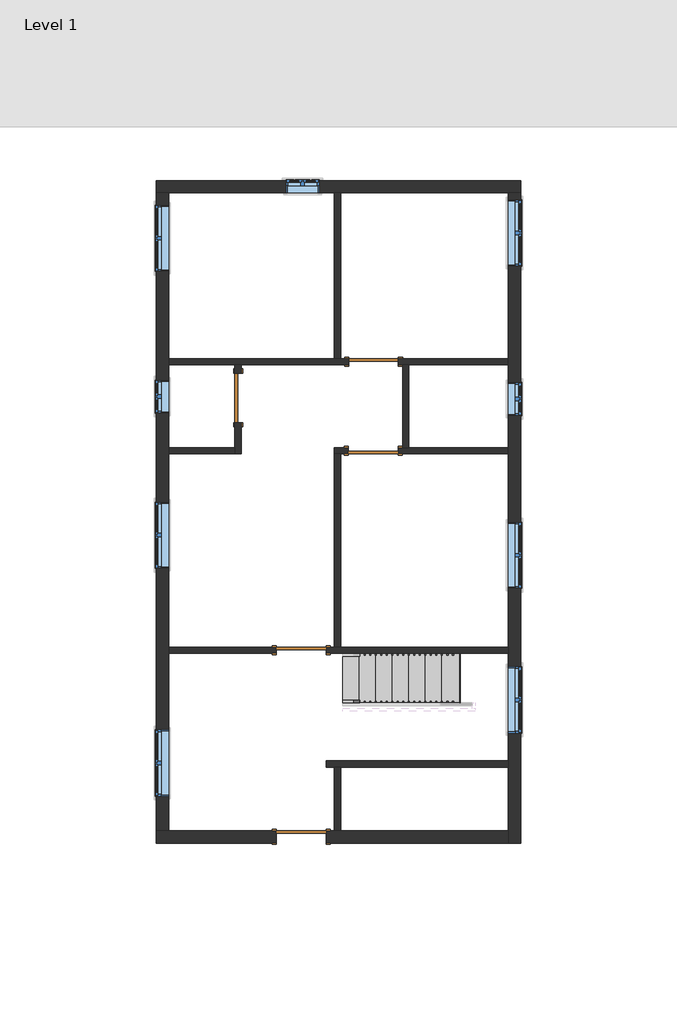
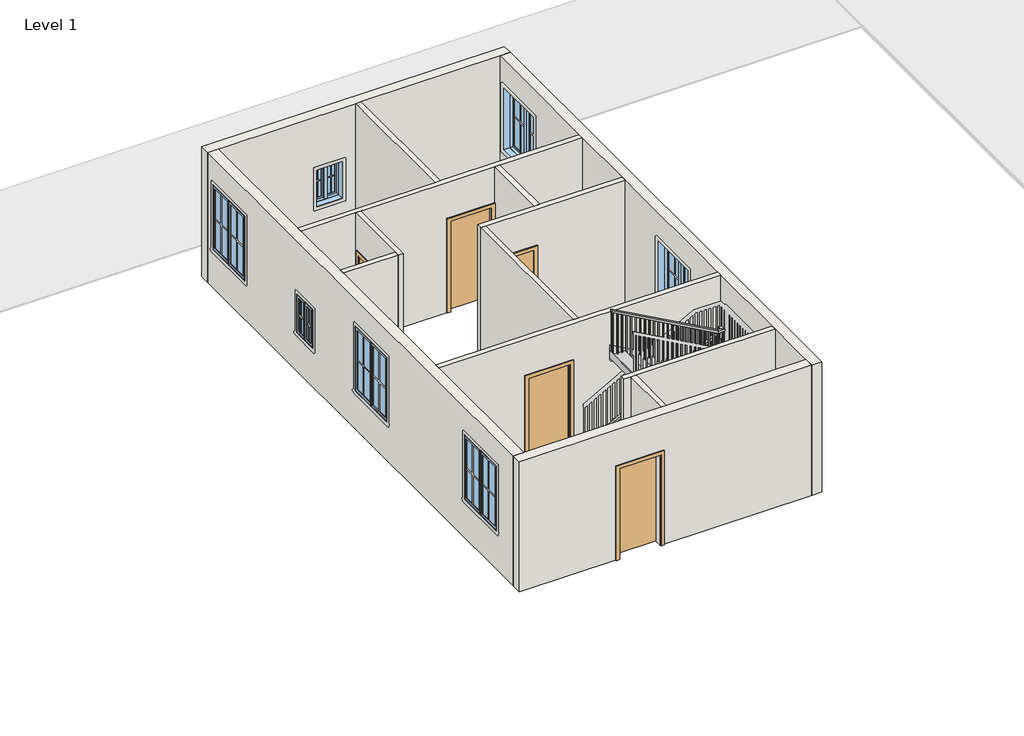
# One storey, part 1 of 2: 14 walls, 9 windows, 5 doors, 1 railing, 1 stair flight.
"""IFC4 building model written with IfcOpenShell, lengths in millimetres."""

from ifc_helpers import new_model, si_unit, frame, origin, origin_with_axes, place, context, project, spatial, polyline, outline, extrude, faceted_brep, transform, mapped, element, save
from components import door_305aa2a5, door_e5f9f3c4, door_a90ba1ad, stair_flight_0ccda8d3, window_c417fced, window_8377141f

model = new_model("IFC4")

# Units and contexts
model_context = context("Model", 3, world=origin())
ifc_project = project(units=[si_unit("LENGTHUNIT", "METRE", prefix="MILLI")], contexts=[model_context])

# Site, building, storey
site = spatial("IfcSite", under=ifc_project)
building = spatial("IfcBuilding", under=site)
storey = spatial("IfcBuildingStorey", under=building, Name="Level 1", Elevation=0.0)

# Doors
placement = place(None, origin())
door_shape = door_305aa2a5(model_context)
element("IfcDoor", 1, ObjectType="Single-Flush : 36\" x 84\"", at=placement, inside=storey, context=model_context, shape_type="MappedRepresentation", body=[
    mapped(door_shape, transform((5270.5, 10636.25, 0.0), x_axis=(-1.0, 0.0, 0.0), y_axis=(0.0, -1.0, 0.0), z_axis=(0.0, 0.0, 1.0))),
])
door_2_shape = door_e5f9f3c4(model_context)
element("IfcDoor", 2, ObjectType="Single-Flush : 36\" x 84\"", at=placement, inside=storey, context=model_context, shape_type="MappedRepresentation", body=[
    mapped(door_2_shape, transform((2774.95, 9969.5, 0.0), x_axis=(0.0, 1.0, 0.0), y_axis=(-1.0, 0.0, 0.0), z_axis=(0.0, 0.0, 1.0))),
])
element("IfcDoor", 3, ObjectType="Single-Flush : 36\" x 84\"", at=placement, inside=storey, context=model_context, shape_type="MappedRepresentation", body=[
    mapped(door_2_shape, transform((5264.15, 8997.95, 0.0), x_axis=(-1.0, 0.0, 0.0), y_axis=(0.0, -1.0, 0.0), z_axis=(0.0, 0.0, 1.0))),
])
element("IfcDoor", 4, ObjectType="Single-Flush : 36\" x 84\"", at=placement, inside=storey, context=model_context, shape_type="MappedRepresentation", body=[
    mapped(door_2_shape, transform((3937.0, 5327.65, 0.0), x_axis=(1.0, 0.0, 0.0), y_axis=(0.0, 1.0, 0.0), z_axis=(0.0, 0.0, 1.0))),
])
door_3_shape = door_a90ba1ad(model_context)
element("IfcDoor", 5, ObjectType="Single-Flush : 36\" x 84\"", at=placement, inside=storey, context=model_context, shape_type="MappedRepresentation", body=[
    mapped(door_3_shape, transform((3937.0, 1892.3, 0.0), x_axis=(-1.0, 0.0, 0.0), y_axis=(0.0, -1.0, 0.0), z_axis=(0.0, 0.0, 1.0))),
])

# Railing
element("IfcRailing", 6, ObjectType="Handrail - Rectangular", at=placement, inside=storey, context=model_context, shape_type="SolidModel", body=[
    faceted_brep([(4699.0, 4406.9, 1083.7333333), (4699.0, 4406.9, 1025.620221), (4699.0, 4356.1, 1025.620221), (4699.0, 4356.1, 1083.7333333), (7061.2, 4406.9, 2396.0666667), (7112.0, 4406.9, 2366.1757765), (7112.0, 4356.1, 2366.1757765), (7061.2, 4356.1, 2396.0666667), (7061.2, 4406.9, 2438.4), (7112.0, 4406.9, 2387.6), (7112.0, 4356.1, 2387.6), (7061.2, 4356.1, 2438.4), (7188.2, 4406.9, 2438.4), (7188.2, 4406.9, 2387.6), (7137.4, 4356.1, 2387.6), (7137.4, 4356.1, 2438.4), (7188.2, 4279.9, 2438.4), (7188.2, 4229.1, 2387.6), (7137.4, 4229.1, 2387.6), (7137.4, 4279.9, 2438.4), (7188.2, 4279.9, 2650.0666667), (7188.2, 4229.1, 2599.2666667), (7137.4, 4229.1, 2599.2666667), (7137.4, 4279.9, 2650.0666667), (7188.2, 4152.9, 2650.0666667), (7188.2, 4152.9, 2599.2666667), (7137.4, 4203.7, 2599.2666667), (7137.4, 4203.7, 2650.0666667), (7061.2, 4152.9, 2650.0666667), (7048.0363978, 4152.9, 2599.2666667), (7048.0363978, 4203.7, 2599.2666667), (7061.2, 4203.7, 2650.0666667), (4699.0, 4152.9, 3962.4), (4699.0, 4203.7, 3962.4), (4699.0, 4203.7, 3904.2868876), (4699.0, 4152.9, 3904.2868876)], [[[0, 1, 2, 3]], [[1, 0, 4, 5]], [[2, 1, 5, 6]], [[3, 2, 6, 7]], [[0, 3, 7, 4]], [[5, 4, 8, 9]], [[6, 5, 9, 10]], [[7, 6, 10, 11]], [[4, 7, 11, 8]], [[9, 8, 12, 13]], [[10, 9, 13, 14]], [[11, 10, 14, 15]], [[8, 11, 15, 12]], [[13, 12, 16, 17]], [[14, 13, 17, 18]], [[15, 14, 18, 19]], [[12, 15, 19, 16]], [[17, 16, 20, 21]], [[18, 17, 21, 22]], [[19, 18, 22, 23]], [[16, 19, 23, 20]], [[21, 20, 24, 25]], [[22, 21, 25, 26]], [[23, 22, 26, 27]], [[20, 23, 27, 24]], [[25, 24, 28, 29]], [[26, 25, 29, 30]], [[27, 26, 30, 31]], [[24, 27, 31, 28]], [[32, 33, 34, 35]], [[29, 28, 32, 35]], [[30, 29, 35, 34]], [[31, 30, 34, 33]], [[28, 31, 33, 32]]]),
    extrude(outline(polyline([(3884.8841099, 4733.925), (3895.4674432, 4714.875), (2878.6666667, 4714.875), (2878.6666667, 4733.925), (3884.8841099, 4733.925)])), frame((0.0, 4168.775, 0.0), z_axis=(0.0, 1.0, 0.0), x_axis=(0.0, 0.0, 1.0)), (0.0, 0.0, 1.0), 19.05),
    extrude(outline(polyline([(3828.4396654, 4835.525), (3839.0229988, 4816.475), (2878.6666667, 4816.475), (2878.6666667, 4835.525), (3828.4396654, 4835.525)])), frame((0.0, 4168.775, 0.0), z_axis=(0.0, 1.0, 0.0), x_axis=(0.0, 0.0, 1.0)), (0.0, 0.0, 1.0), 19.05),
    extrude(outline(polyline([(3771.995221, 4937.125), (3782.5785543, 4918.075), (2878.6666667, 4918.075), (2878.6666667, 4937.125), (3771.995221, 4937.125)])), frame((0.0, 4168.775, 0.0), z_axis=(0.0, 1.0, 0.0), x_axis=(0.0, 0.0, 1.0)), (0.0, 0.0, 1.0), 19.05),
    extrude(outline(polyline([(3715.5507765, 5038.725), (3726.1341099, 5019.675), (2709.3333333, 5019.675), (2709.3333333, 5038.725), (3715.5507765, 5038.725)])), frame((0.0, 4168.775, 0.0), z_axis=(0.0, 1.0, 0.0), x_axis=(0.0, 0.0, 1.0)), (0.0, 0.0, 1.0), 19.05),
    extrude(outline(polyline([(3659.1063321, 5140.325), (3669.6896654, 5121.275), (2709.3333333, 5121.275), (2709.3333333, 5140.325), (3659.1063321, 5140.325)])), frame((0.0, 4168.775, 0.0), z_axis=(0.0, 1.0, 0.0), x_axis=(0.0, 0.0, 1.0)), (0.0, 0.0, 1.0), 19.05),
    extrude(outline(polyline([(3602.6618876, 5241.925), (3613.245221, 5222.875), (2709.3333333, 5222.875), (2709.3333333, 5241.925), (3602.6618876, 5241.925)])), frame((0.0, 4168.775, 0.0), z_axis=(0.0, 1.0, 0.0), x_axis=(0.0, 0.0, 1.0)), (0.0, 0.0, 1.0), 19.05),
    extrude(outline(polyline([(3546.2174432, 5343.525), (3556.8007765, 5324.475), (2540.0, 5324.475), (2540.0, 5343.525), (3546.2174432, 5343.525)])), frame((0.0, 4168.775, 0.0), z_axis=(0.0, 1.0, 0.0), x_axis=(0.0, 0.0, 1.0)), (0.0, 0.0, 1.0), 19.05),
    extrude(outline(polyline([(3489.7729988, 5445.125), (3500.3563321, 5426.075), (2540.0, 5426.075), (2540.0, 5445.125), (3489.7729988, 5445.125)])), frame((0.0, 4168.775, 0.0), z_axis=(0.0, 1.0, 0.0), x_axis=(0.0, 0.0, 1.0)), (0.0, 0.0, 1.0), 19.05),
    extrude(outline(polyline([(3433.3285543, 5546.725), (3443.9118876, 5527.675), (2540.0, 5527.675), (2540.0, 5546.725), (3433.3285543, 5546.725)])), frame((0.0, 4168.775, 0.0), z_axis=(0.0, 1.0, 0.0), x_axis=(0.0, 0.0, 1.0)), (0.0, 0.0, 1.0), 19.05),
    extrude(outline(polyline([(3376.8841099, 5648.325), (3387.4674432, 5629.275), (2370.6666667, 5629.275), (2370.6666667, 5648.325), (3376.8841099, 5648.325)])), frame((0.0, 4168.775, 0.0), z_axis=(0.0, 1.0, 0.0), x_axis=(0.0, 0.0, 1.0)), (0.0, 0.0, 1.0), 19.05),
    extrude(outline(polyline([(3320.4396654, 5749.925), (3331.0229988, 5730.875), (2370.6666667, 5730.875), (2370.6666667, 5749.925), (3320.4396654, 5749.925)])), frame((0.0, 4168.775, 0.0), z_axis=(0.0, 1.0, 0.0), x_axis=(0.0, 0.0, 1.0)), (0.0, 0.0, 1.0), 19.05),
    extrude(outline(polyline([(3263.995221, 5851.525), (3274.5785543, 5832.475), (2370.6666667, 5832.475), (2370.6666667, 5851.525), (3263.995221, 5851.525)])), frame((0.0, 4168.775, 0.0), z_axis=(0.0, 1.0, 0.0), x_axis=(0.0, 0.0, 1.0)), (0.0, 0.0, 1.0), 19.05),
    extrude(outline(polyline([(3207.5507765, 5953.125), (3218.1341099, 5934.075), (2201.3333333, 5934.075), (2201.3333333, 5953.125), (3207.5507765, 5953.125)])), frame((0.0, 4168.775, 0.0), z_axis=(0.0, 1.0, 0.0), x_axis=(0.0, 0.0, 1.0)), (0.0, 0.0, 1.0), 19.05),
    extrude(outline(polyline([(3151.1063321, 6054.725), (3161.6896654, 6035.675), (2201.3333333, 6035.675), (2201.3333333, 6054.725), (3151.1063321, 6054.725)])), frame((0.0, 4168.775, 0.0), z_axis=(0.0, 1.0, 0.0), x_axis=(0.0, 0.0, 1.0)), (0.0, 0.0, 1.0), 19.05),
    extrude(outline(polyline([(3094.6618876, 6156.325), (3105.245221, 6137.275), (2201.3333333, 6137.275), (2201.3333333, 6156.325), (3094.6618876, 6156.325)])), frame((0.0, 4168.775, 0.0), z_axis=(0.0, 1.0, 0.0), x_axis=(0.0, 0.0, 1.0)), (0.0, 0.0, 1.0), 19.05),
    extrude(outline(polyline([(3038.2174432, 6257.925), (3048.8007765, 6238.875), (2032.0, 6238.875), (2032.0, 6257.925), (3038.2174432, 6257.925)])), frame((0.0, 4168.775, 0.0), z_axis=(0.0, 1.0, 0.0), x_axis=(0.0, 0.0, 1.0)), (0.0, 0.0, 1.0), 19.05),
    extrude(outline(polyline([(2981.7729988, 6359.525), (2992.3563321, 6340.475), (2032.0, 6340.475), (2032.0, 6359.525), (2981.7729988, 6359.525)])), frame((0.0, 4168.775, 0.0), z_axis=(0.0, 1.0, 0.0), x_axis=(0.0, 0.0, 1.0)), (0.0, 0.0, 1.0), 19.05),
    extrude(outline(polyline([(2925.3285543, 6461.125), (2935.9118876, 6442.075), (2032.0, 6442.075), (2032.0, 6461.125), (2925.3285543, 6461.125)])), frame((0.0, 4168.775, 0.0), z_axis=(0.0, 1.0, 0.0), x_axis=(0.0, 0.0, 1.0)), (0.0, 0.0, 1.0), 19.05),
    extrude(outline(polyline([(2868.8841099, 6562.725), (2879.4674432, 6543.675), (1862.6666667, 6543.675), (1862.6666667, 6562.725), (2868.8841099, 6562.725)])), frame((0.0, 4168.775, 0.0), z_axis=(0.0, 1.0, 0.0), x_axis=(0.0, 0.0, 1.0)), (0.0, 0.0, 1.0), 19.05),
    extrude(outline(polyline([(2812.4396654, 6664.325), (2823.0229988, 6645.275), (1862.6666667, 6645.275), (1862.6666667, 6664.325), (2812.4396654, 6664.325)])), frame((0.0, 4168.775, 0.0), z_axis=(0.0, 1.0, 0.0), x_axis=(0.0, 0.0, 1.0)), (0.0, 0.0, 1.0), 19.05),
    extrude(outline(polyline([(2755.995221, 6765.925), (2766.5785543, 6746.875), (1862.6666667, 6746.875), (1862.6666667, 6765.925), (2755.995221, 6765.925)])), frame((0.0, 4168.775, 0.0), z_axis=(0.0, 1.0, 0.0), x_axis=(0.0, 0.0, 1.0)), (0.0, 0.0, 1.0), 19.05),
    extrude(outline(polyline([(2699.5507765, 6867.525), (2710.1341099, 6848.475), (1693.3333333, 6848.475), (1693.3333333, 6867.525), (2699.5507765, 6867.525)])), frame((0.0, 4168.775, 0.0), z_axis=(0.0, 1.0, 0.0), x_axis=(0.0, 0.0, 1.0)), (0.0, 0.0, 1.0), 19.05),
    extrude(outline(polyline([(2643.1063321, 6969.125), (2653.6896654, 6950.075), (1693.3333333, 6950.075), (1693.3333333, 6969.125), (2643.1063321, 6969.125)])), frame((0.0, 4168.775, 0.0), z_axis=(0.0, 1.0, 0.0), x_axis=(0.0, 0.0, 1.0)), (0.0, 0.0, 1.0), 19.05),
    extrude(outline(polyline([(2586.6618876, 7070.725), (2597.245221, 7051.675), (1693.3333333, 7051.675), (1693.3333333, 7070.725), (2586.6618876, 7070.725)])), frame((0.0, 4168.775, 0.0), z_axis=(0.0, 1.0, 0.0), x_axis=(0.0, 0.0, 1.0)), (0.0, 0.0, 1.0), 19.05),
    extrude(outline(polyline([(7153.275, 4289.425), (7172.325, 4289.425), (7172.325, 4270.375), (7153.275, 4270.375), (7153.275, 4289.425)])), frame((0.0, 0.0, 1524.0), z_axis=(0.0, 0.0, 1.0), x_axis=(1.0, 0.0, 0.0)), (0.0, 0.0, 1.0), 863.6),
    extrude(outline(polyline([(7127.875, 4371.975), (7127.875, 4391.025), (7146.925, 4391.025), (7146.925, 4371.975), (7127.875, 4371.975)])), frame((0.0, 0.0, 1524.0), z_axis=(0.0, 0.0, 1.0), x_axis=(1.0, 0.0, 0.0)), (0.0, 0.0, 1.0), 863.6),
    extrude(outline(polyline([(2329.1341099, 7045.325), (2318.5507765, 7026.275), (1354.6666667, 7026.275), (1354.6666667, 7045.325), (2329.1341099, 7045.325)])), frame((0.0, 4371.975, 0.0), z_axis=(0.0, 1.0, 0.0), x_axis=(0.0, 0.0, 1.0)), (0.0, 0.0, 1.0), 19.05),
    extrude(outline(polyline([(2272.6896654, 6943.725), (2262.1063321, 6924.675), (1354.6666667, 6924.675), (1354.6666667, 6943.725), (2272.6896654, 6943.725)])), frame((0.0, 4371.975, 0.0), z_axis=(0.0, 1.0, 0.0), x_axis=(0.0, 0.0, 1.0)), (0.0, 0.0, 1.0), 19.05),
    extrude(outline(polyline([(2216.245221, 6842.125), (2205.6618876, 6823.075), (1354.6666667, 6823.075), (1354.6666667, 6842.125), (2216.245221, 6842.125)])), frame((0.0, 4371.975, 0.0), z_axis=(0.0, 1.0, 0.0), x_axis=(0.0, 0.0, 1.0)), (0.0, 0.0, 1.0), 19.05),
    extrude(outline(polyline([(2159.8007765, 6740.525), (2149.2174432, 6721.475), (1185.3333333, 6721.475), (1185.3333333, 6740.525), (2159.8007765, 6740.525)])), frame((0.0, 4371.975, 0.0), z_axis=(0.0, 1.0, 0.0), x_axis=(0.0, 0.0, 1.0)), (0.0, 0.0, 1.0), 19.05),
    extrude(outline(polyline([(2103.3563321, 6638.925), (2092.7729988, 6619.875), (1185.3333333, 6619.875), (1185.3333333, 6638.925), (2103.3563321, 6638.925)])), frame((0.0, 4371.975, 0.0), z_axis=(0.0, 1.0, 0.0), x_axis=(0.0, 0.0, 1.0)), (0.0, 0.0, 1.0), 19.05),
    extrude(outline(polyline([(2046.9118876, 6537.325), (2036.3285543, 6518.275), (1185.3333333, 6518.275), (1185.3333333, 6537.325), (2046.9118876, 6537.325)])), frame((0.0, 4371.975, 0.0), z_axis=(0.0, 1.0, 0.0), x_axis=(0.0, 0.0, 1.0)), (0.0, 0.0, 1.0), 19.05),
    extrude(outline(polyline([(1990.4674432, 6435.725), (1979.8841099, 6416.675), (1016.0, 6416.675), (1016.0, 6435.725), (1990.4674432, 6435.725)])), frame((0.0, 4371.975, 0.0), z_axis=(0.0, 1.0, 0.0), x_axis=(0.0, 0.0, 1.0)), (0.0, 0.0, 1.0), 19.05),
    extrude(outline(polyline([(1934.0229988, 6334.125), (1923.4396654, 6315.075), (1016.0, 6315.075), (1016.0, 6334.125), (1934.0229988, 6334.125)])), frame((0.0, 4371.975, 0.0), z_axis=(0.0, 1.0, 0.0), x_axis=(0.0, 0.0, 1.0)), (0.0, 0.0, 1.0), 19.05),
    extrude(outline(polyline([(1877.5785543, 6232.525), (1866.995221, 6213.475), (1016.0, 6213.475), (1016.0, 6232.525), (1877.5785543, 6232.525)])), frame((0.0, 4371.975, 0.0), z_axis=(0.0, 1.0, 0.0), x_axis=(0.0, 0.0, 1.0)), (0.0, 0.0, 1.0), 19.05),
    extrude(outline(polyline([(1821.1341099, 6130.925), (1810.5507765, 6111.875), (846.6666667, 6111.875), (846.6666667, 6130.925), (1821.1341099, 6130.925)])), frame((0.0, 4371.975, 0.0), z_axis=(0.0, 1.0, 0.0), x_axis=(0.0, 0.0, 1.0)), (0.0, 0.0, 1.0), 19.05),
    extrude(outline(polyline([(1764.6896654, 6029.325), (1754.1063321, 6010.275), (846.6666667, 6010.275), (846.6666667, 6029.325), (1764.6896654, 6029.325)])), frame((0.0, 4371.975, 0.0), z_axis=(0.0, 1.0, 0.0), x_axis=(0.0, 0.0, 1.0)), (0.0, 0.0, 1.0), 19.05),
    extrude(outline(polyline([(1708.245221, 5927.725), (1697.6618876, 5908.675), (846.6666667, 5908.675), (846.6666667, 5927.725), (1708.245221, 5927.725)])), frame((0.0, 4371.975, 0.0), z_axis=(0.0, 1.0, 0.0), x_axis=(0.0, 0.0, 1.0)), (0.0, 0.0, 1.0), 19.05),
    extrude(outline(polyline([(1651.8007765, 5826.125), (1641.2174432, 5807.075), (677.3333333, 5807.075), (677.3333333, 5826.125), (1651.8007765, 5826.125)])), frame((0.0, 4371.975, 0.0), z_axis=(0.0, 1.0, 0.0), x_axis=(0.0, 0.0, 1.0)), (0.0, 0.0, 1.0), 19.05),
    extrude(outline(polyline([(1595.3563321, 5724.525), (1584.7729988, 5705.475), (677.3333333, 5705.475), (677.3333333, 5724.525), (1595.3563321, 5724.525)])), frame((0.0, 4371.975, 0.0), z_axis=(0.0, 1.0, 0.0), x_axis=(0.0, 0.0, 1.0)), (0.0, 0.0, 1.0), 19.05),
    extrude(outline(polyline([(1538.9118876, 5622.925), (1528.3285543, 5603.875), (677.3333333, 5603.875), (677.3333333, 5622.925), (1538.9118876, 5622.925)])), frame((0.0, 4371.975, 0.0), z_axis=(0.0, 1.0, 0.0), x_axis=(0.0, 0.0, 1.0)), (0.0, 0.0, 1.0), 19.05),
    extrude(outline(polyline([(1482.4674432, 5521.325), (1471.8841099, 5502.275), (508.0, 5502.275), (508.0, 5521.325), (1482.4674432, 5521.325)])), frame((0.0, 4371.975, 0.0), z_axis=(0.0, 1.0, 0.0), x_axis=(0.0, 0.0, 1.0)), (0.0, 0.0, 1.0), 19.05),
    extrude(outline(polyline([(1426.0229988, 5419.725), (1415.4396654, 5400.675), (508.0, 5400.675), (508.0, 5419.725), (1426.0229988, 5419.725)])), frame((0.0, 4371.975, 0.0), z_axis=(0.0, 1.0, 0.0), x_axis=(0.0, 0.0, 1.0)), (0.0, 0.0, 1.0), 19.05),
    extrude(outline(polyline([(1369.5785543, 5318.125), (1358.995221, 5299.075), (508.0, 5299.075), (508.0, 5318.125), (1369.5785543, 5318.125)])), frame((0.0, 4371.975, 0.0), z_axis=(0.0, 1.0, 0.0), x_axis=(0.0, 0.0, 1.0)), (0.0, 0.0, 1.0), 19.05),
    extrude(outline(polyline([(1313.1341099, 5216.525), (1302.5507765, 5197.475), (338.6666667, 5197.475), (338.6666667, 5216.525), (1313.1341099, 5216.525)])), frame((0.0, 4371.975, 0.0), z_axis=(0.0, 1.0, 0.0), x_axis=(0.0, 0.0, 1.0)), (0.0, 0.0, 1.0), 19.05),
    extrude(outline(polyline([(1256.6896654, 5114.925), (1246.1063321, 5095.875), (338.6666667, 5095.875), (338.6666667, 5114.925), (1256.6896654, 5114.925)])), frame((0.0, 4371.975, 0.0), z_axis=(0.0, 1.0, 0.0), x_axis=(0.0, 0.0, 1.0)), (0.0, 0.0, 1.0), 19.05),
    extrude(outline(polyline([(1200.245221, 5013.325), (1189.6618876, 4994.275), (338.6666667, 4994.275), (338.6666667, 5013.325), (1200.245221, 5013.325)])), frame((0.0, 4371.975, 0.0), z_axis=(0.0, 1.0, 0.0), x_axis=(0.0, 0.0, 1.0)), (0.0, 0.0, 1.0), 19.05),
    extrude(outline(polyline([(1143.8007765, 4911.725), (1133.2174432, 4892.675), (169.3333333, 4892.675), (169.3333333, 4911.725), (1143.8007765, 4911.725)])), frame((0.0, 4371.975, 0.0), z_axis=(0.0, 1.0, 0.0), x_axis=(0.0, 0.0, 1.0)), (0.0, 0.0, 1.0), 19.05),
    extrude(outline(polyline([(1087.3563321, 4810.125), (1076.7729988, 4791.075), (169.3333333, 4791.075), (169.3333333, 4810.125), (1087.3563321, 4810.125)])), frame((0.0, 4371.975, 0.0), z_axis=(0.0, 1.0, 0.0), x_axis=(0.0, 0.0, 1.0)), (0.0, 0.0, 1.0), 19.05),
    extrude(outline(polyline([(7153.275, 4187.825), (7172.325, 4187.825), (7172.325, 4168.775), (7153.275, 4168.775), (7153.275, 4187.825)])), frame((0.0, 0.0, 1524.0), z_axis=(0.0, 0.0, 1.0), x_axis=(1.0, 0.0, 0.0)), (0.0, 0.0, 1.0), 1075.2666667),
    extrude(outline(polyline([(7153.275, 4371.975), (7153.275, 4391.025), (7172.325, 4391.025), (7172.325, 4371.975), (7153.275, 4371.975)])), frame((0.0, 0.0, 1524.0), z_axis=(0.0, 0.0, 1.0), x_axis=(1.0, 0.0, 0.0)), (0.0, 0.0, 1.0), 863.6),
    extrude(outline(polyline([(3893.7035543, 4718.05), (3904.2868876, 4699.0), (2878.6666667, 4699.0), (2878.6666667, 4718.05), (3893.7035543, 4718.05)])), frame((0.0, 4168.775, 0.0), z_axis=(0.0, 1.0, 0.0), x_axis=(0.0, 0.0, 1.0)), (0.0, 0.0, 1.0), 19.05),
    extrude(outline(polyline([(1036.2035543, 4718.05), (1025.620221, 4699.0), (169.3333333, 4699.0), (169.3333333, 4718.05), (1036.2035543, 4718.05)])), frame((0.0, 4371.975, 0.0), z_axis=(0.0, 1.0, 0.0), x_axis=(0.0, 0.0, 1.0)), (0.0, 0.0, 1.0), 19.05),
])

# Stair flight
stair_flight_shape = stair_flight_0ccda8d3(model_context)
element("IfcStairFlight", 7, ObjectType="2\" Tread 1\" Nosing 1/4\" Riser", at=placement, inside=storey, context=model_context, shape_type="MappedRepresentation", body=[
    mapped(stair_flight_shape, transform((0.0, 0.0, 0.0), x_axis=(1.0, 0.0, 0.0), y_axis=(0.0, 1.0, 0.0), z_axis=(0.0, 0.0, 1.0))),
])

# Walls
element("IfcWall", 8, ObjectType="Generic - 5\"", at=placement, inside=storey, context=model_context, shape_type="SweptSolid", body=[
    extrude(outline(polyline([(4546.6, 10693.4), (4546.6, 13741.4), (4660.9, 13741.4), (4660.9, 10693.4), (4546.6, 10693.4)])), origin_with_axes(), (0.0, 0.0, 1.0), 3048.0),
])
element("IfcWall", 9, ObjectType="Generic - 5\"", at=placement, inside=storey, context=model_context, shape_type="Brep", body=[
    faceted_brep([(1498.6, 10579.1, 0.0), (2717.8, 10579.1, 0.0), (2832.1, 10579.1, 0.0), (4813.3, 10579.1, 0.0), (4813.3, 10579.1, 2133.6), (5727.7, 10579.1, 2133.6), (5727.7, 10579.1, 0.0), (5803.9, 10579.1, 0.0), (5918.2, 10579.1, 0.0), (7747.0, 10579.1, 0.0), (7747.0, 10579.1, 3048.0), (5918.2, 10579.1, 3048.0), (5803.9, 10579.1, 3048.0), (2832.1, 10579.1, 3048.0), (2717.8, 10579.1, 3048.0), (1498.6, 10579.1, 3048.0), (4813.3, 10693.4, 2133.6), (4813.3, 10693.4, 0.0), (4660.9, 10693.4, 0.0), (4546.6, 10693.4, 0.0), (1498.6, 10693.4, 0.0), (1498.6, 10693.4, 3048.0), (4546.6, 10693.4, 3048.0), (4660.9, 10693.4, 3048.0), (7747.0, 10693.4, 3048.0), (7747.0, 10693.4, 0.0), (5727.7, 10693.4, 0.0), (5727.7, 10693.4, 2133.6)], [[[0, 1, 2, 3, 4, 5, 6, 7, 8, 9, 10, 11, 12, 13, 14, 15]], [[16, 17, 18, 19, 20, 21, 22, 23, 24, 25, 26, 27]], [[26, 25, 9, 8, 7, 6]], [[20, 19, 18, 17, 3, 2, 1, 0]], [[15, 14, 13, 12, 11, 10, 24, 23, 22, 21]], [[10, 9, 25, 24]], [[0, 15, 21, 20]], [[4, 3, 17, 16]], [[5, 4, 16, 27]], [[6, 5, 27, 26]]]),
])
element("IfcWall", 10, ObjectType="Generic - 5\"", at=placement, inside=storey, context=model_context, shape_type="Brep", body=[
    faceted_brep([(2717.8, 10579.1, 0.0), (2717.8, 10426.7, 0.0), (2717.8, 10426.7, 2133.6), (2717.8, 9512.3, 2133.6), (2717.8, 9512.3, 0.0), (2717.8, 9055.1, 0.0), (2717.8, 8940.8, 0.0), (2717.8, 8940.8, 3048.0), (2717.8, 9055.1, 3048.0), (2717.8, 10579.1, 3048.0), (2832.1, 10426.7, 2133.6), (2832.1, 10426.7, 0.0), (2832.1, 10579.1, 0.0), (2832.1, 10579.1, 3048.0), (2832.1, 8940.8, 3048.0), (2832.1, 8940.8, 0.0), (2832.1, 9512.3, 0.0), (2832.1, 9512.3, 2133.6)], [[[0, 1, 2, 3, 4, 5, 6, 7, 8, 9]], [[10, 11, 12, 13, 14, 15, 16, 17]], [[16, 15, 6, 5, 4]], [[12, 11, 1, 0]], [[9, 8, 7, 14, 13]], [[0, 9, 13, 12]], [[7, 6, 15, 14]], [[2, 1, 11, 10]], [[3, 2, 10, 17]], [[4, 3, 17, 16]]]),
])
element("IfcWall", 11, ObjectType="Generic - 5\"", at=placement, inside=storey, context=model_context, shape_type="SweptSolid", body=[
    extrude(outline(polyline([(2717.8, 8940.8), (1498.6, 8940.8), (1498.6, 9055.1), (2717.8, 9055.1), (2717.8, 8940.8)])), origin_with_axes(), (0.0, 0.0, 1.0), 3048.0),
])
element("IfcWall", 12, ObjectType="Generic - 5\"", at=placement, inside=storey, context=model_context, shape_type="SweptSolid", body=[
    extrude(outline(polyline([(5803.9, 9055.1), (5803.9, 10579.1), (5918.2, 10579.1), (5918.2, 9055.1), (5803.9, 9055.1)])), origin_with_axes(), (0.0, 0.0, 1.0), 3048.0),
])
element("IfcWall", 13, ObjectType="Generic - 5\"", at=placement, inside=storey, context=model_context, shape_type="Brep", body=[
    faceted_brep([(4806.95, 9055.1, 2133.6), (4806.95, 9055.1, 0.0), (4546.6, 9055.1, 0.0), (4546.6, 9055.1, 3048.0), (5803.9, 9055.1, 3048.0), (5918.2, 9055.1, 3048.0), (7747.0, 9055.1, 3048.0), (7747.0, 9055.1, 0.0), (5918.2, 9055.1, 0.0), (5803.9, 9055.1, 0.0), (5721.35, 9055.1, 0.0), (5721.35, 9055.1, 2133.6), (4546.6, 8940.8, 0.0), (4660.9, 8940.8, 0.0), (4806.95, 8940.8, 0.0), (4806.95, 8940.8, 2133.6), (5721.35, 8940.8, 2133.6), (5721.35, 8940.8, 0.0), (7747.0, 8940.8, 0.0), (7747.0, 8940.8, 3048.0), (4660.9, 8940.8, 3048.0), (4546.6, 8940.8, 3048.0)], [[[0, 1, 2, 3, 4, 5, 6, 7, 8, 9, 10, 11]], [[12, 13, 14, 15, 16, 17, 18, 19, 20, 21]], [[2, 1, 14, 13, 12]], [[10, 9, 8, 7, 18, 17]], [[6, 5, 4, 3, 21, 20, 19]], [[7, 6, 19, 18]], [[3, 2, 12, 21]], [[15, 14, 1, 0]], [[16, 15, 0, 11]], [[17, 16, 11, 10]]]),
])
element("IfcWall", 14, ObjectType="Generic - 5\"", at=placement, inside=storey, context=model_context, shape_type="Brep", body=[
    faceted_brep([(4394.2, 5270.5, 2133.6), (4394.2, 5270.5, 0.0), (7747.0, 5270.5, 0.0), (7747.0, 5270.5, 3048.0), (1498.6, 5270.5, 3048.0), (1498.6, 5270.5, 0.0), (3479.8, 5270.5, 0.0), (3479.8, 5270.5, 2133.6), (7747.0, 5384.8, 0.0), (4660.9, 5384.8, 0.0), (4546.6, 5384.8, 0.0), (4394.2, 5384.8, 0.0), (4394.2, 5384.8, 2133.6), (3479.8, 5384.8, 2133.6), (3479.8, 5384.8, 0.0), (1498.6, 5384.8, 0.0), (1498.6, 5384.8, 3048.0), (4546.6, 5384.8, 3048.0), (4660.9, 5384.8, 3048.0), (7747.0, 5384.8, 3048.0)], [[[0, 1, 2, 3, 4, 5, 6, 7]], [[8, 9, 10, 11, 12, 13, 14, 15, 16, 17, 18, 19]], [[6, 5, 15, 14]], [[2, 1, 11, 10, 9, 8]], [[4, 3, 19, 18, 17, 16]], [[3, 2, 8, 19]], [[5, 4, 16, 15]], [[12, 11, 1, 0]], [[13, 12, 0, 7]], [[14, 13, 7, 6]]]),
])
element("IfcWall", 15, ObjectType="Generic - 5\"", at=placement, inside=storey, context=model_context, shape_type="SweptSolid", body=[
    extrude(outline(polyline([(4660.9, 8940.8), (4660.9, 5384.8), (4546.6, 5384.8), (4546.6, 8940.8), (4660.9, 8940.8)])), origin_with_axes(), (0.0, 0.0, 1.0), 3048.0),
])
element("IfcWall", 16, ObjectType="Generic - 5\"", at=placement, inside=storey, context=model_context, shape_type="SweptSolid", body=[
    extrude(outline(polyline([(4660.9, 3175.0), (4660.9, 2006.6), (4546.6, 2006.6), (4546.6, 3175.0), (4660.9, 3175.0)])), origin_with_axes(), (0.0, 0.0, 1.0), 3048.0),
])
element("IfcWall", 17, ObjectType="Generic - 5\"", at=placement, inside=storey, context=model_context, shape_type="Brep", body=[
    faceted_brep([(4394.2, 3175.0, 0.0), (4546.6, 3175.0, 0.0), (4660.9, 3175.0, 0.0), (7747.0, 3175.0, 0.0), (7747.0, 3175.0, 3048.0), (4660.9, 3175.0, 3048.0), (4546.6, 3175.0, 3048.0), (4394.2, 3175.0, 3048.0), (4394.2, 3289.3, 0.0), (4394.2, 3289.3, 3048.0), (7747.0, 3289.3, 3048.0), (7747.0, 3289.3, 0.0)], [[[0, 1, 2, 3, 4, 5, 6, 7]], [[8, 9, 10, 11]], [[3, 2, 1, 0, 8, 11]], [[7, 6, 5, 4, 10, 9]], [[0, 7, 9, 8]], [[4, 3, 11, 10]]]),
])
element("IfcWall", 18, ObjectType="Generic - 8\"", at=placement, inside=storey, context=model_context, shape_type="Brep", body=[
    faceted_brep([(1270.0, 13741.4, 0.0), (1498.6, 13741.4, 0.0), (4546.6, 13741.4, 0.0), (4660.9, 13741.4, 0.0), (7747.0, 13741.4, 0.0), (7975.6, 13741.4, 0.0), (7975.6, 13741.4, 3048.0), (7747.0, 13741.4, 3048.0), (4660.9, 13741.4, 3048.0), (4546.6, 13741.4, 3048.0), (1498.6, 13741.4, 3048.0), (1270.0, 13741.4, 3048.0), (4267.2, 13741.4, 1828.8), (4267.2, 13741.4, 914.4), (3657.6, 13741.4, 914.4), (3657.6, 13741.4, 1828.8), (1270.0, 13970.0, 0.0), (1270.0, 13970.0, 3048.0), (7975.6, 13970.0, 3048.0), (7975.6, 13970.0, 0.0), (4267.2, 13970.0, 1828.8), (3657.6, 13970.0, 1828.8), (3657.6, 13970.0, 914.4), (4267.2, 13970.0, 914.4)], [[[0, 1, 2, 3, 4, 5, 6, 7, 8, 9, 10, 11], [12, 13, 14, 15]], [[16, 17, 18, 19], [20, 21, 22, 23]], [[5, 4, 3, 2, 1, 0, 16, 19]], [[6, 5, 19, 18]], [[0, 11, 17, 16]], [[13, 12, 20, 23]], [[14, 13, 23, 22]], [[15, 14, 22, 21]], [[12, 15, 21, 20]], [[11, 10, 9, 8, 7, 6, 18, 17]]]),
])
element("IfcWall", 19, ObjectType="Generic - 8\"", at=placement, inside=storey, context=model_context, shape_type="Brep", body=[
    faceted_brep([(7747.0, 13741.4, 0.0), (7747.0, 10693.4, 0.0), (7747.0, 10579.1, 0.0), (7747.0, 9055.1, 0.0), (7747.0, 8940.8, 0.0), (7747.0, 5384.8, 0.0), (7747.0, 5270.5, 0.0), (7747.0, 3289.3, 0.0), (7747.0, 3175.0, 0.0), (7747.0, 2006.6, 0.0), (7747.0, 1778.0, 0.0), (7747.0, 1778.0, 3048.0), (7747.0, 2006.6, 3048.0), (7747.0, 3175.0, 3048.0), (7747.0, 3289.3, 3048.0), (7747.0, 5270.5, 3048.0), (7747.0, 5384.8, 3048.0), (7747.0, 8940.8, 3048.0), (7747.0, 9055.1, 3048.0), (7747.0, 10579.1, 3048.0), (7747.0, 10693.4, 3048.0), (7747.0, 13741.4, 3048.0), (7747.0, 12395.2, 2438.4), (7747.0, 12395.2, 914.4), (7747.0, 13614.4, 914.4), (7747.0, 13614.4, 2438.4), (7747.0, 6464.3, 2438.4), (7747.0, 6464.3, 914.4), (7747.0, 7683.5, 914.4), (7747.0, 7683.5, 2438.4), (7747.0, 9645.65, 1828.8), (7747.0, 9645.65, 914.4), (7747.0, 10255.25, 914.4), (7747.0, 10255.25, 1828.8), (7747.0, 3803.65, 2438.4), (7747.0, 3803.65, 914.4), (7747.0, 5022.85, 914.4), (7747.0, 5022.85, 2438.4), (7975.6, 13741.4, 0.0), (7975.6, 13741.4, 3048.0), (7975.6, 1778.0, 3048.0), (7975.6, 1778.0, 0.0), (7975.6, 12395.2, 2438.4), (7975.6, 13614.4, 2438.4), (7975.6, 13614.4, 914.4), (7975.6, 12395.2, 914.4), (7975.6, 6464.3, 2438.4), (7975.6, 7683.5, 2438.4), (7975.6, 7683.5, 914.4), (7975.6, 6464.3, 914.4), (7975.6, 9645.65, 1828.8), (7975.6, 10255.25, 1828.8), (7975.6, 10255.25, 914.4), (7975.6, 9645.65, 914.4), (7975.6, 3803.65, 2438.4), (7975.6, 5022.85, 2438.4), (7975.6, 5022.85, 914.4), (7975.6, 3803.65, 914.4)], [[[0, 1, 2, 3, 4, 5, 6, 7, 8, 9, 10, 11, 12, 13, 14, 15, 16, 17, 18, 19, 20, 21], [22, 23, 24, 25], [26, 27, 28, 29], [30, 31, 32, 33], [34, 35, 36, 37]], [[38, 39, 40, 41], [42, 43, 44, 45], [46, 47, 48, 49], [50, 51, 52, 53], [54, 55, 56, 57]], [[10, 9, 8, 7, 6, 5, 4, 3, 2, 1, 0, 38, 41]], [[0, 21, 39, 38]], [[11, 10, 41, 40]], [[23, 22, 42, 45]], [[24, 23, 45, 44]], [[25, 24, 44, 43]], [[22, 25, 43, 42]], [[27, 26, 46, 49]], [[28, 27, 49, 48]], [[29, 28, 48, 47]], [[26, 29, 47, 46]], [[31, 30, 50, 53]], [[32, 31, 53, 52]], [[33, 32, 52, 51]], [[30, 33, 51, 50]], [[35, 34, 54, 57]], [[36, 35, 57, 56]], [[37, 36, 56, 55]], [[34, 37, 55, 54]], [[21, 20, 19, 18, 17, 16, 15, 14, 13, 12, 11, 40, 39]]]),
])
element("IfcWall", 20, ObjectType="Generic - 8\"", at=placement, inside=storey, context=model_context, shape_type="Brep", body=[
    faceted_brep([(3479.8, 2006.6, 2133.6), (3479.8, 2006.6, 0.0), (1498.6, 2006.6, 0.0), (1270.0, 2006.6, 0.0), (1270.0, 2006.6, 3048.0), (1498.6, 2006.6, 3048.0), (4546.6, 2006.6, 3048.0), (4660.9, 2006.6, 3048.0), (7747.0, 2006.6, 3048.0), (7747.0, 2006.6, 0.0), (4660.9, 2006.6, 0.0), (4546.6, 2006.6, 0.0), (4394.2, 2006.6, 0.0), (4394.2, 2006.6, 2133.6), (1270.0, 1778.0, 0.0), (3479.8, 1778.0, 0.0), (3479.8, 1778.0, 2133.6), (4394.2, 1778.0, 2133.6), (4394.2, 1778.0, 0.0), (7747.0, 1778.0, 0.0), (7747.0, 1778.0, 3048.0), (1270.0, 1778.0, 3048.0)], [[[0, 1, 2, 3, 4, 5, 6, 7, 8, 9, 10, 11, 12, 13]], [[14, 15, 16, 17, 18, 19, 20, 21]], [[3, 2, 1, 15, 14]], [[12, 11, 10, 9, 19, 18]], [[9, 8, 20, 19]], [[4, 3, 14, 21]], [[16, 15, 1, 0]], [[17, 16, 0, 13]], [[18, 17, 13, 12]], [[8, 7, 6, 5, 4, 21, 20]]]),
])
element("IfcWall", 21, ObjectType="Generic - 8\"", at=placement, inside=storey, context=model_context, shape_type="Brep", body=[
    faceted_brep([(1498.6, 2006.6, 0.0), (1498.6, 5270.5, 0.0), (1498.6, 5384.8, 0.0), (1498.6, 8940.8, 0.0), (1498.6, 9055.1, 0.0), (1498.6, 10579.1, 0.0), (1498.6, 10693.4, 0.0), (1498.6, 13741.4, 0.0), (1498.6, 13741.4, 3048.0), (1498.6, 10693.4, 3048.0), (1498.6, 10579.1, 3048.0), (1498.6, 9055.1, 3048.0), (1498.6, 8940.8, 3048.0), (1498.6, 5384.8, 3048.0), (1498.6, 5270.5, 3048.0), (1498.6, 2006.6, 3048.0), (1498.6, 3860.3039063, 2438.4), (1498.6, 3860.3039063, 914.4), (1498.6, 2641.1039063, 914.4), (1498.6, 2641.1039063, 2438.4), (1498.6, 8054.4789062, 2438.4), (1498.6, 8054.4789062, 914.4), (1498.6, 6835.2789062, 914.4), (1498.6, 6835.2789062, 2438.4), (1498.6, 13518.6539062, 2438.4), (1498.6, 13518.6539062, 914.4), (1498.6, 12299.4539062, 914.4), (1498.6, 12299.4539062, 2438.4), (1498.6, 10299.2039062, 1828.8), (1498.6, 10299.2039062, 914.4), (1498.6, 9689.6039062, 914.4), (1498.6, 9689.6039062, 1828.8), (1270.0, 2006.6, 0.0), (1270.0, 2006.6, 3048.0), (1270.0, 13741.4, 3048.0), (1270.0, 13741.4, 0.0), (1270.0, 3860.3039063, 2438.4), (1270.0, 2641.1039063, 2438.4), (1270.0, 2641.1039063, 914.4), (1270.0, 3860.3039063, 914.4), (1270.0, 8054.4789062, 2438.4), (1270.0, 6835.2789062, 2438.4), (1270.0, 6835.2789062, 914.4), (1270.0, 8054.4789062, 914.4), (1270.0, 13518.6539062, 2438.4), (1270.0, 12299.4539062, 2438.4), (1270.0, 12299.4539062, 914.4), (1270.0, 13518.6539062, 914.4), (1270.0, 10299.2039062, 1828.8), (1270.0, 9689.6039062, 1828.8), (1270.0, 9689.6039062, 914.4), (1270.0, 10299.2039062, 914.4)], [[[0, 1, 2, 3, 4, 5, 6, 7, 8, 9, 10, 11, 12, 13, 14, 15], [16, 17, 18, 19], [20, 21, 22, 23], [24, 25, 26, 27], [28, 29, 30, 31]], [[32, 33, 34, 35], [36, 37, 38, 39], [40, 41, 42, 43], [44, 45, 46, 47], [48, 49, 50, 51]], [[7, 6, 5, 4, 3, 2, 1, 0, 32, 35]], [[0, 15, 33, 32]], [[8, 7, 35, 34]], [[17, 16, 36, 39]], [[18, 17, 39, 38]], [[19, 18, 38, 37]], [[16, 19, 37, 36]], [[21, 20, 40, 43]], [[22, 21, 43, 42]], [[23, 22, 42, 41]], [[20, 23, 41, 40]], [[25, 24, 44, 47]], [[26, 25, 47, 46]], [[27, 26, 46, 45]], [[24, 27, 45, 44]], [[29, 28, 48, 51]], [[30, 29, 51, 50]], [[31, 30, 50, 49]], [[28, 31, 49, 48]], [[15, 14, 13, 12, 11, 10, 9, 8, 34, 33]]]),
])

# Windows
window_shape = window_c417fced(model_context)
element("IfcWindow", 22, ObjectType="Window-Casement-Double : 24\" x 36\"", at=placement, inside=storey, context=model_context, shape_type="MappedRepresentation", body=[
    mapped(window_shape, transform((3962.4, 13855.7, 0.0), x_axis=(1.0, 0.0, 0.0), y_axis=(0.0, 1.0, 0.0), z_axis=(0.0, 0.0, 1.0))),
])
element("IfcWindow", 23, ObjectType="Window-Casement-Double : 24\" x 36\"", at=placement, inside=storey, context=model_context, shape_type="MappedRepresentation", body=[
    mapped(window_shape, transform((7861.3, 9950.45, 0.0), x_axis=(0.0, -1.0, 0.0), y_axis=(1.0, 0.0, 0.0), z_axis=(0.0, 0.0, 1.0))),
])
element("IfcWindow", 24, ObjectType="Window-Casement-Double : 24\" x 36\"", at=placement, inside=storey, context=model_context, shape_type="MappedRepresentation", body=[
    mapped(window_shape, transform((1384.3, 9994.4039062, 0.0), x_axis=(0.0, 1.0, 0.0), y_axis=(-1.0, 0.0, 0.0), z_axis=(0.0, 0.0, 1.0))),
])
window_2_shape = window_8377141f(model_context)
element("IfcWindow", 25, ObjectType="Window-Casement-Double : 48\" x 60\"", at=placement, inside=storey, context=model_context, shape_type="MappedRepresentation", body=[
    mapped(window_2_shape, transform((1384.3, 3250.7039063, 0.0), x_axis=(0.0, 1.0, 0.0), y_axis=(-1.0, 0.0, 0.0), z_axis=(0.0, 0.0, 1.0))),
])
element("IfcWindow", 26, ObjectType="Window-Casement-Double : 48\" x 60\"", at=placement, inside=storey, context=model_context, shape_type="MappedRepresentation", body=[
    mapped(window_2_shape, transform((1384.3, 7444.8789063, 0.0), x_axis=(0.0, 1.0, 0.0), y_axis=(-1.0, 0.0, 0.0), z_axis=(0.0, 0.0, 1.0))),
])
element("IfcWindow", 27, ObjectType="Window-Casement-Double : 48\" x 60\"", at=placement, inside=storey, context=model_context, shape_type="MappedRepresentation", body=[
    mapped(window_2_shape, transform((1384.3, 12909.0539063, 0.0), x_axis=(0.0, 1.0, 0.0), y_axis=(-1.0, 0.0, 0.0), z_axis=(0.0, 0.0, 1.0))),
])
element("IfcWindow", 28, ObjectType="Window-Casement-Double : 48\" x 60\"", at=placement, inside=storey, context=model_context, shape_type="MappedRepresentation", body=[
    mapped(window_2_shape, transform((7861.3, 13004.8, 0.0), x_axis=(0.0, -1.0, 0.0), y_axis=(1.0, 0.0, 0.0), z_axis=(0.0, 0.0, 1.0))),
])
element("IfcWindow", 29, ObjectType="Window-Casement-Double : 48\" x 60\"", at=placement, inside=storey, context=model_context, shape_type="MappedRepresentation", body=[
    mapped(window_2_shape, transform((7861.3, 7073.9, 0.0), x_axis=(0.0, -1.0, 0.0), y_axis=(1.0, 0.0, 0.0), z_axis=(0.0, 0.0, 1.0))),
])
element("IfcWindow", 30, ObjectType="Window-Casement-Double : 48\" x 60\"", at=placement, inside=storey, context=model_context, shape_type="MappedRepresentation", body=[
    mapped(window_2_shape, transform((7861.3, 4413.25, 0.0), x_axis=(0.0, -1.0, 0.0), y_axis=(1.0, 0.0, 0.0), z_axis=(0.0, 0.0, 1.0))),
])

save(model, "model.ifc")

# Revit data of these elements
# Type "Single-Flush : 36\" x 84\""
#   Type Mark = "1"
#   Construction Type Id = "MDOOR"
#   Assembly Code = "C1020"
#   Analytic Construction = "Metal"
#   Thickness = 0' - 2"
#   Heat Transfer Coefficient (U) = 0.651978 BTU/(h·ft²·°F)
#   Height = 7' - 0"
#   Trim Projection Ext = 0' - 1"
#   Trim Projection Int = 0' - 1"
#   Trim Width = 0' - 3"
#   Width = 3' - 0"
#   Define Thermal Properties by = 1
#   Define Thermal Properties by = 1
#   Door Material = Door - Panel
#   Frame Material = Door - Frame
#   Visual Light Transmittance = 0
#   Solar Heat Gain Coefficient = 0
#   Function = (empty or 0)
#   Wall Closure = (empty or 0)
# Type "Handrail - Rectangular"
#   Assembly Code = "C2010400"
#   built-in parameter 1008612 = 0.0416667 (stored number, unit not read)
#   built-in parameter 1008611 = 0.0416667 (stored number, unit not read)
#   built-in parameter 1008609 = 0.333333 (stored number, unit not read)
#   built-in parameter 1008604 = 0.166667 (stored number, unit not read)
#   built-in parameter 1008603 = 0.166667 (stored number, unit not read)
#   Railing Height = 3' - 0"
#   built-in parameter 1008630 = 2
#   built-in parameter 1008610 = 2
#   built-in parameter 1008618 = Baluster - Square : 3/4"
# Type "Generic - 5\""
#   Assembly Code = "B2010"
#   Layers, outside or top first: 0' - 4 1/2" no material (function 1)
# Type "Generic - 8\""
#   Assembly Code = "B2010"
#   Layers, outside or top first: 0' - 9" no material (function 1)
# Type "Window-Casement-Double : 24\" x 36\""
#   Type Mark = "14"
#   Fire Rating = "0.5h"
#   Assembly Code = "B2020100"
#   Analytic Construction = "Double glazing - domestic"
#   Frame Extension [instance default] = 0' - 0 1/4"
#   Window Inset [instance default] = 0' - 0"
#   Wall Thickness [instance default] = 0' - 6"
#   Interior Wall Closure [instance default] = 0' - 2 1/4"
#   Half Width = 1' - 0"
#   Visual Light Transmittance = 0.81
#   Thermal Resistance (R) = 1.8146 (h·ft²·°F)/BTU
#   Solar Heat Gain Coefficient = 0.76
#   Rough Width = 2' - 0 1/2"
#   Rough Height = 3' - 0 1/2"
#   Height = 3' - 0"
#   Heat Transfer Coefficient (U) = 0.5511 BTU/(h·ft²·°F)
#   Exterior Wall Closure [instance default] = 0' - 1 1/4"
#   Extension Jamb [instance default] = 0' - 2 1/4"
#   Default Sill Height = 3' - 0"
#   Width = 2' - 0"
#   Define Thermal Properties by = 0
#   Muntin Visibility = yes
#   Interior Trim Visibility [instance default] = yes
#   Exterior Trim Visibility [instance default] = yes
#   Extension Jamb Visibility [instance default] = yes
#   Interior Trim Material = Wood - Stained
#   Muntin Pattern = Muntin Pattern_2x2 : Muntin Pattern_2x2
#   Interior Trim = Trim-Window-Interior-Flat : Picture Frame
#   Interior Frame Material = Wood - Stained
#   Glass Panel Material = Glass
#   Exterior Trim Material = Clad - White
#   Exterior Trim = Trim-Window-Exterior-Flat : with Sill
#   Exterior Frame Material = Clad - White
#   Wall Closure = (empty or 0)
# Type "Window-Casement-Double : 48\" x 60\""
#   Type Mark = "17"
#   Fire Rating = "0.5h"
#   Assembly Code = "B2020100"
#   Analytic Construction = "Double glazing - domestic"
#   Frame Extension [instance default] = 0' - 0 1/4"
#   Window Inset [instance default] = 0' - 0"
#   Wall Thickness [instance default] = 0' - 6"
#   Interior Wall Closure [instance default] = 0' - 2 1/4"
#   Half Width = 2' - 0"
#   Visual Light Transmittance = 0.81
#   Thermal Resistance (R) = 1.8146 (h·ft²·°F)/BTU
#   Solar Heat Gain Coefficient = 0.76
#   Rough Width = 4' - 0 1/2"
#   Rough Height = 5' - 0 1/2"
#   Height = 5' - 0"
#   Heat Transfer Coefficient (U) = 0.5511 BTU/(h·ft²·°F)
#   Exterior Wall Closure [instance default] = 0' - 1 1/4"
#   Extension Jamb [instance default] = 0' - 2 1/4"
#   Default Sill Height = 3' - 0"
#   Width = 4' - 0"
#   Define Thermal Properties by = 0
#   Muntin Visibility = yes
#   Interior Trim Visibility [instance default] = yes
#   Exterior Trim Visibility [instance default] = yes
#   Extension Jamb Visibility [instance default] = yes
#   Interior Trim Material = Wood - Stained
#   Muntin Pattern = Muntin Pattern_2x2 : Muntin Pattern_2x2
#   Interior Trim = Trim-Window-Interior-Flat : Picture Frame
#   Interior Frame Material = Wood - Stained
#   Glass Panel Material = Glass
#   Exterior Trim Material = Clad - White
#   Exterior Trim = Trim-Window-Exterior-Flat : with Sill
#   Exterior Frame Material = Clad - White
#   Wall Closure = (empty or 0)
# Elements 1, 2, 3, 4, 5 (IfcDoor, "Single-Flush : 36\" x 84\"")
#   Phase Created = New Construction
#   Materials on its faces: "Door - Frame", "Door - Panel"
# Element 6 (IfcRailing, "Handrail - Rectangular")
#   Phase Created = New Construction
# Element 7 (IfcStairFlight, "2\" Tread 1\" Nosing 1/4\" Riser")
#   Phase Created = New Construction
# Elements 8, 9, 10, 11, 12, 13, 14, 15, 16, 17 (IfcWall, "Generic - 5\"")
#   Top Offset = 0' - 0"
#   Base Offset = 0' - 0"
#   wall height = 10' - 0"
#   Phase Created = New Construction
#   Base Constraint = Level 1
#   Top Constraint = Level 2
#   Materials on its faces: "Default Wall"
# Elements 18, 19, 20, 21 (IfcWall, "Generic - 8\"")
#   Top Offset = 0' - 0"
#   Base Offset = 0' - 0"
#   Unconnected Height = 10' - 0"
#   wall height = 10' - 0"
#   Phase Created = New Construction
#   Base Constraint = Level 1
#   Materials on its faces: "Default Wall", "Wood - Stained"
# Element 22 (IfcWindow, "Window-Casement-Double : 24\" x 36\"")
#   Mark = "6"
#   Window Inset = 0' - 0"
#   Interior Wall Closure = 0' - 2 1/4"
#   Frame Extension = 0' - 0 1/4"
#   Exterior Wall Closure = 0' - 1 1/4"
#   Interior Trim Visibility = yes
#   Exterior Trim Visibility = yes
#   Phase Created = New Construction
#   Materials on its faces: "Wood - Stained", "Glass", "Clad - White"
# Element 23 (IfcWindow, "Window-Casement-Double : 24\" x 36\"")
#   Mark = "7"
#   Window Inset = 0' - 0"
#   Interior Wall Closure = 0' - 2 1/4"
#   Frame Extension = 0' - 0 1/4"
#   Exterior Wall Closure = 0' - 1 1/4"
#   Interior Trim Visibility = yes
#   Exterior Trim Visibility = yes
#   Phase Created = New Construction
#   Materials on its faces: "Wood - Stained", "Glass", "Clad - White"
# Element 24 (IfcWindow, "Window-Casement-Double : 24\" x 36\"")
#   Mark = "8"
#   Window Inset = 0' - 0"
#   Interior Wall Closure = 0' - 2 1/4"
#   Frame Extension = 0' - 0 1/4"
#   Exterior Wall Closure = 0' - 1 1/4"
#   Interior Trim Visibility = yes
#   Exterior Trim Visibility = yes
#   Phase Created = New Construction
#   Materials on its faces: "Wood - Stained", "Glass", "Clad - White"
# Element 25 (IfcWindow, "Window-Casement-Double : 48\" x 60\"")
#   Mark = "1"
#   Window Inset = 0' - 0"
#   Interior Wall Closure = 0' - 2 1/4"
#   Frame Extension = 0' - 0 1/4"
#   Exterior Wall Closure = 0' - 1 1/4"
#   Interior Trim Visibility = yes
#   Exterior Trim Visibility = yes
#   Phase Created = New Construction
#   Materials on its faces: "Wood - Stained", "Glass", "Clad - White"
# Element 26 (IfcWindow, "Window-Casement-Double : 48\" x 60\"")
#   Mark = "2"
#   Window Inset = 0' - 0"
#   Interior Wall Closure = 0' - 2 1/4"
#   Frame Extension = 0' - 0 1/4"
#   Exterior Wall Closure = 0' - 1 1/4"
#   Interior Trim Visibility = yes
#   Exterior Trim Visibility = yes
#   Phase Created = New Construction
#   Materials on its faces: "Wood - Stained", "Glass", "Clad - White"
# Element 27 (IfcWindow, "Window-Casement-Double : 48\" x 60\"")
#   Mark = "3"
#   Window Inset = 0' - 0"
#   Interior Wall Closure = 0' - 2 1/4"
#   Frame Extension = 0' - 0 1/4"
#   Exterior Wall Closure = 0' - 1 1/4"
#   Interior Trim Visibility = yes
#   Exterior Trim Visibility = yes
#   Phase Created = New Construction
#   Materials on its faces: "Wood - Stained", "Glass", "Clad - White"
# Element 28 (IfcWindow, "Window-Casement-Double : 48\" x 60\"")
#   Mark = "4"
#   Window Inset = 0' - 0"
#   Interior Wall Closure = 0' - 2 1/4"
#   Frame Extension = 0' - 0 1/4"
#   Exterior Wall Closure = 0' - 1 1/4"
#   Interior Trim Visibility = yes
#   Exterior Trim Visibility = yes
#   Phase Created = New Construction
#   Materials on its faces: "Wood - Stained", "Glass", "Clad - White"
# Element 29 (IfcWindow, "Window-Casement-Double : 48\" x 60\"")
#   Mark = "5"
#   Window Inset = 0' - 0"
#   Interior Wall Closure = 0' - 2 1/4"
#   Frame Extension = 0' - 0 1/4"
#   Exterior Wall Closure = 0' - 1 1/4"
#   Interior Trim Visibility = yes
#   Exterior Trim Visibility = yes
#   Phase Created = New Construction
#   Materials on its faces: "Wood - Stained", "Glass", "Clad - White"
# Element 30 (IfcWindow, "Window-Casement-Double : 48\" x 60\"")
#   Mark = "10"
#   Window Inset = 0' - 0"
#   Interior Wall Closure = 0' - 2 1/4"
#   Frame Extension = 0' - 0 1/4"
#   Exterior Wall Closure = 0' - 1 1/4"
#   Interior Trim Visibility = yes
#   Exterior Trim Visibility = yes
#   Phase Created = New Construction
#   Materials on its faces: "Wood - Stained", "Glass", "Clad - White"
# Materials
#   "Door - Panel": class "Wood", colour RGB 210 159 95, transparency 0, Cost = 0
#   "Door - Frame": colour RGB 118 70 51, transparency 0, Cost = 0
#   "Wood - Stained": class "Wood", colour RGB 224 178 126, transparency 0, Cost = 0
#   "Glass": class "Glass", colour RGB 0 128 192, transparency 0.75, Description = "Soda Lime Glass", Cost = 0
#   "Clad - White": class "Wood", colour RGB 242 242 238, transparency 0, Cost = 0
#   "Default Wall": colour RGB 128 128 128, transparency 0, Cost = 0
